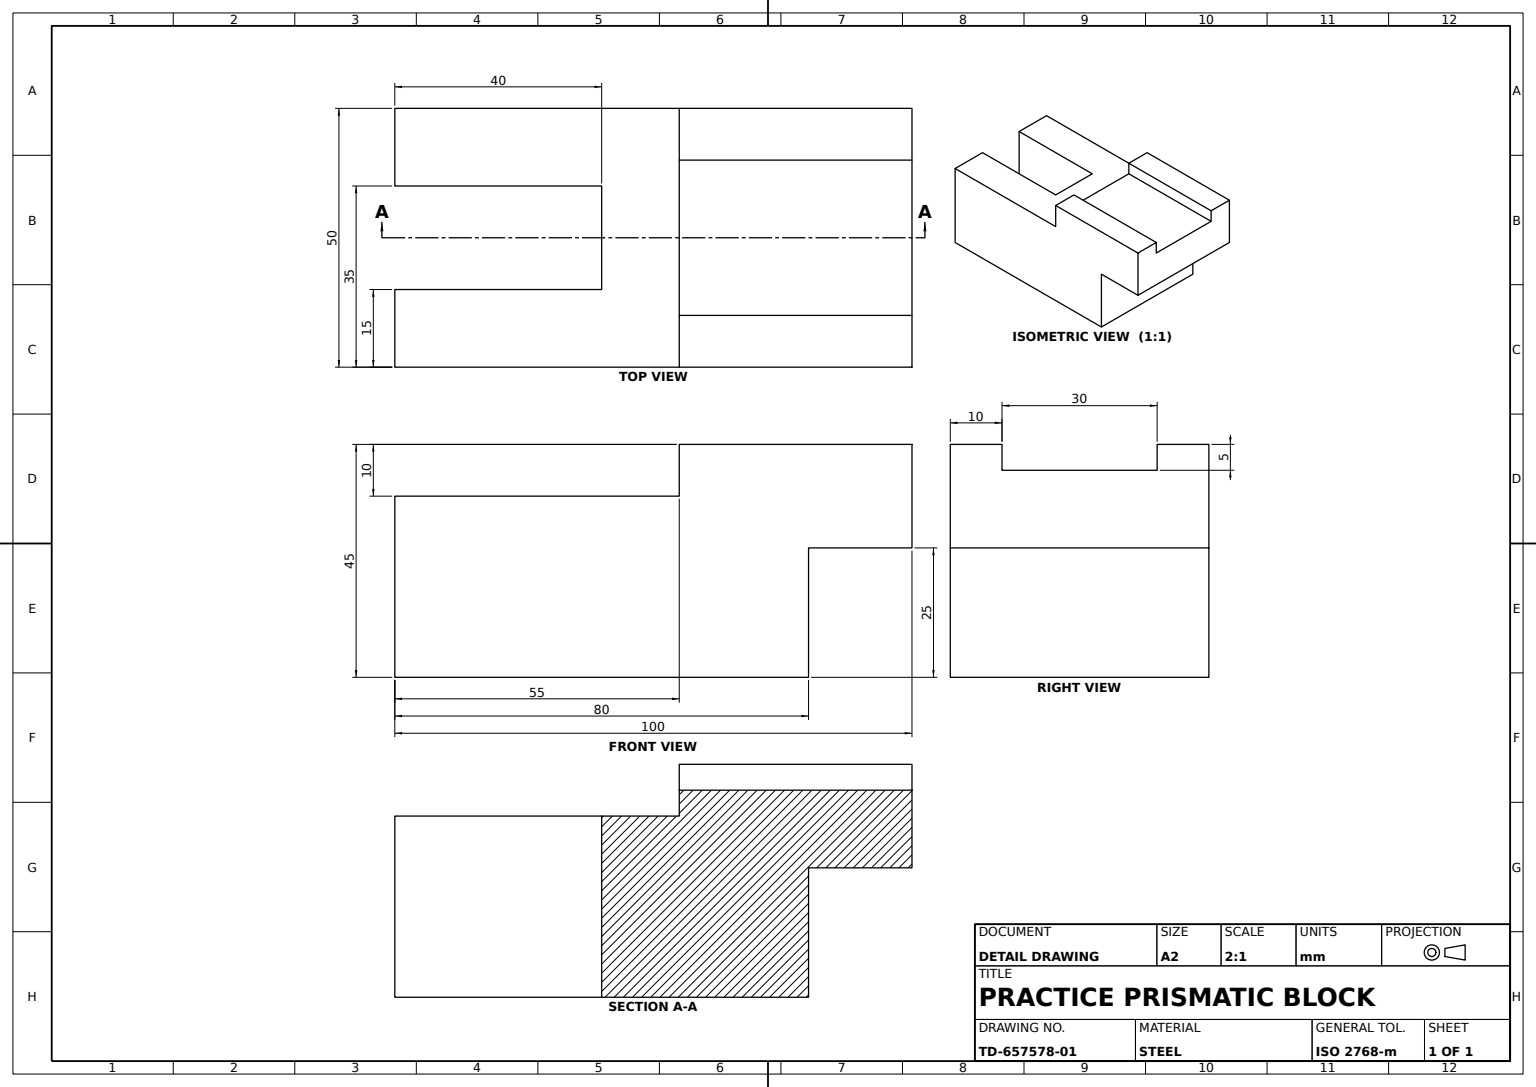
SolidWorks part; units mm, degrees
material "Plain Carbon Steel"
ref_plane "Front Plane" through (0, 0, 0) normal (0, 0, 1) x (1, 0, 0)
ref_plane "Top Plane" through (0, 0, 0) normal (0, 1, 0) x (1, 0, 0)
ref_plane "Right Plane" through (0, 0, 0) normal (1, 0, 0) x (0, 0, -1)
sketch "Base Block Profile" plane through (0, 0, 0) normal (0, 0, 1) x (1, 0, 0)
  line L0 (0, 0) -> (80, 0)
  line L1 (80, 0) -> (80, 25)
  line L2 (80, 25) -> (100, 25)
  line L3 (100, 25) -> (100, 45)
  line L4 (100, 45) -> (55, 45)
  line L5 (55, 45) -> (55, 35)
  line L6 (55, 35) -> (0, 35)
  line L7 (0, 35) -> (0, 0)
  dimension "D1" = 80
  dimension "D2" = 10
  dimension "D3" = 25
  dimension "D4" = 20
  dimension "D5" = 55
  dimension "D6" = 45
extrude "Base Block" add sketch "Base Block Profile" along normal blind 50
sketch "Pocket Profile" plane through (0, 0, 0) normal (-1, 0, 0) x (0, 0, 1)
  line L0 (15, 0) -> (15, 35)
  line L1 (50, 0) -> (0, 0) construction
  line L2 (15, 35) -> (35, 35)
  line L3 (35, 35) -> (35, 0)
  line L4 (35, 0) -> (15, 0)
  line L5 (50, 35) -> (50, 0) construction
  line L6 (0, 35) -> (0, 0) construction
  dimension "D1" = 15
  dimension "D2" = 15
  dimension "D3" = 35
extrude "Rectangular Pocket" cut sketch "Pocket Profile" against normal blind 40
sketch "Slot Profile" plane through (55, 0, 0) normal (-1, 0, 0) x (0, 0, 1)
  line L0 (10, 45) -> (10, 40)
  line L1 (50, 45) -> (0, 45) construction
  line L2 (10, 40) -> (40, 40)
  line L3 (40, 40) -> (40, 45)
  line L4 (40, 45) -> (10, 45)
  line L5 (50, 45) -> (50, 35) construction
  dimension "D1" = 30
  dimension "D2" = 10
  dimension "D3" = 5
extrude "Rectangular Slot" cut sketch "Slot Profile" against normal through all
